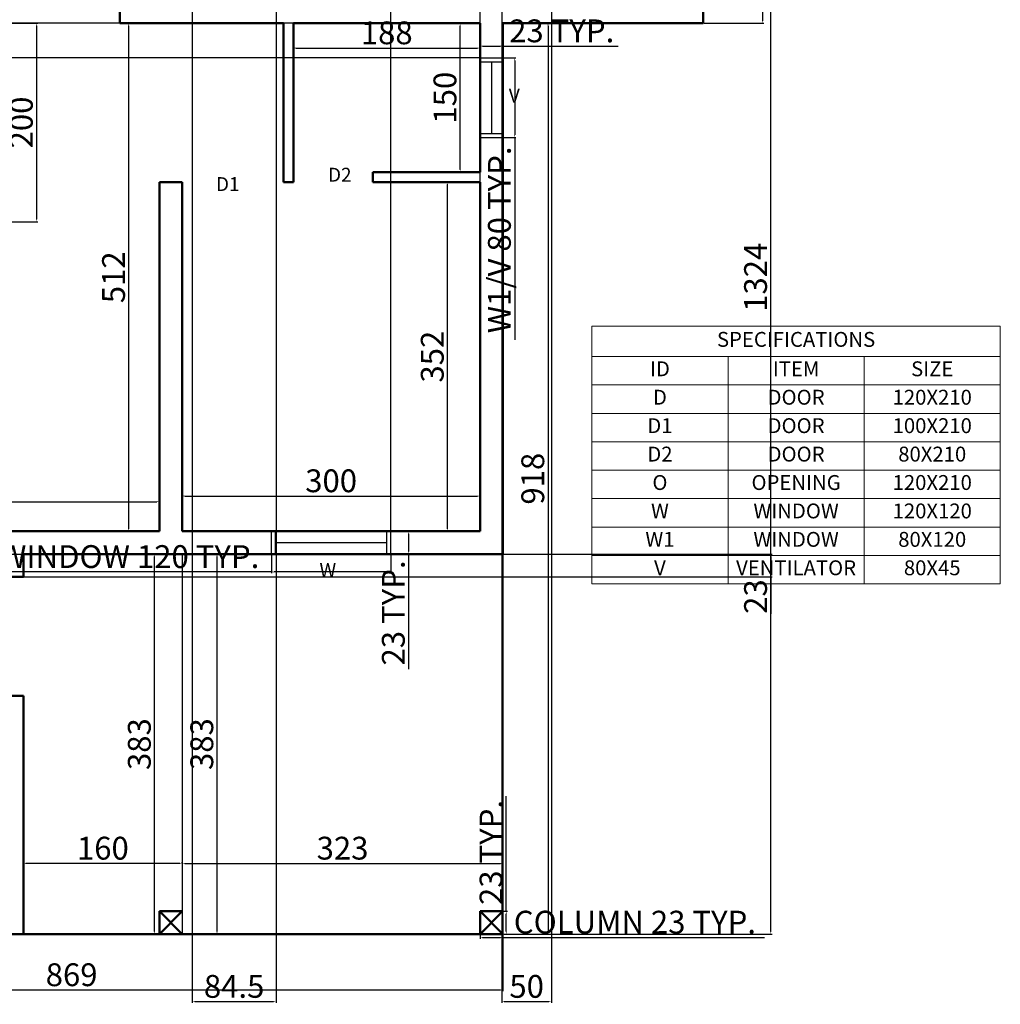
# Model space of a CAD drawing. Units: centimetres. Extents: x 6294 to 7898, y 3240 to 4730.
# Tile 2 of 3: x 6910 to 7898, y 3240 to 4232. Entities that reach past the tile are written whole.
import ezdxf

# ---------------------------------------------------------------- set-up
doc = ezdxf.new("R2010")
doc.units = ezdxf.units.CM
for name, color, linetype, lineweight in [('A-ANNO-DIMS', 2, 'Continuous', 18), ('A-ANNO-SCHD', 7, 'Continuous', 18), ('A-ANNO-TEXT', 7, 'Continuous', 25), ('A-COLS', 7, 'Continuous', 50), ('A-FLOR', 8, 'Continuous', 25), ('A-GLAZ', 4, 'Continuous', 25), ('A-WALL', 7, 'Continuous', 50)]:
    doc.layers.add(name, color=color, linetype=linetype, lineweight=lineweight)
doc.styles.get("Standard").update_dxf_attribs({"font": 'arial.ttf'})
doc.dimstyles.new('ISO-25', dxfattribs={"dimtxt": 23, "dimasz": 2.5, "dimexe": 1.25, "dimexo": 0.625, "dimtad": 1, "dimtxsty": 'Standard', "dimcen": 2.5, "dimadec": 0, "dimazin": 0, "dimtfac": 1, "dimtmove": 0, "dimatfit": 3, "dimfxl": 1, "dimarcsym": 0})

# ---------------------------------------------------------------- blocks, each defined once
blk = doc.blocks.new('*T1')
at = {"layer": 'A-ANNO-SCHD', "transparency": 16777216}
for p, q in [((0, 0), (411.54, 0)), ((0, 0), (0, -259.86)), ((411.54, 0), (411.54, -259.86)), ((0, -30.65), (411.54, -30.65)), ((137.18, -30.65), (137.18, -259.86)), ((274.36, -30.65), (274.36, -259.86)), ((0, -59.3), (411.54, -59.3)), ((0, -87.95), (411.54, -87.95)), ((0, -116.6), (411.54, -116.6)), ((0, -145.25), (411.54, -145.25)), ((0, -173.9), (411.54, -173.9)), ((0, -202.55), (411.54, -202.55)), ((0, -231.2), (411.54, -231.2)), ((0, -259.86), (411.54, -259.86))]:
    blk.add_line(p, q, dxfattribs=at)
at = {"layer": 'A-ANNO-SCHD', "color": 0, "transparency": 16777216, "char_height": 15, "attachment_point": 5}
for s, insert, width in [('SPECIFICATIONS', (205.77, -15.33), 408.5389), ('ID', (68.59, -44.98), 134.1796), ('ITEM', (205.77, -44.98), 134.1796), ('SIZE', (342.95, -44.98), 134.1796), ('D ', (68.59, -73.63), 134.1796), ('DOOR', (205.77, -73.63), 134.1796), ('120X210', (342.95, -73.63), 134.1796), ('D1', (68.59, -102.28), 134.1796), ('DOOR', (205.77, -102.28), 134.1796), ('100X210', (342.95, -102.28), 134.1796), ('D2', (68.59, -130.93), 134.1796), ('DOOR', (205.77, -130.93), 134.1796), ('80X210', (342.95, -130.93), 134.1796), ('O', (68.59, -159.58), 134.1796), ('OPENING', (205.77, -159.58), 134.1796), ('120X210', (342.95, -159.58), 134.1796), ('WINDOW', (205.77, -188.23), 134.1796), ('120X120', (342.95, -188.23), 134.1796), ('W', (68.59, -188.23), 134.1796), ('W1', (68.59, -216.88), 134.1796), ('WINDOW', (205.77, -216.88), 134.1796), ('80X120', (342.95, -216.88), 134.1796), ('V', (68.59, -245.53), 134.1796), ('VENTILATOR', (205.77, -245.53), 134.1796), ('80X45', (342.95, -245.53), 134.1796)]:
    blk.add_mtext(s, dxfattribs=dict(at, insert=insert, width=width))
blk = doc.blocks.new('*D10')
at = {"layer": 'A-ANNO-DIMS', "color": 0, "lineweight": -2, "transparency": 16777216}
for p, q in [((7185.73, 4228.22), (7185.73, 4202.61)), ((7373.73, 4228.22), (7373.73, 4202.61)), ((7188.23, 4203.86), (7371.23, 4203.86))]:
    blk.add_line(p, q, dxfattribs=at)
at = {"layer": 'A-ANNO-DIMS', "color": 0, "transparency": 16777216}
for points in [[(7188.23, 4204.28), (7188.23, 4203.45), (7185.73, 4203.86)], [(7371.23, 4204.28), (7371.23, 4203.45), (7373.73, 4203.86)]]:
    blk.add_solid(points, dxfattribs=at)
at = {"layer": 'Defpoints', "color": 0, "transparency": 16777216}
for p in [(7185.73, 4228.85), (7373.73, 4228.85), (7373.73, 4203.86)]:
    blk.add_point(p, dxfattribs=at)
at = {"layer": 'A-ANNO-DIMS', "color": 0, "transparency": 16777216, "insert": (7279.73, 4216.23), "char_height": 23, "attachment_point": 5}
blk.add_mtext('188', dxfattribs=at)
blk = doc.blocks.new('*D11')
at = {"layer": 'A-ANNO-DIMS', "color": 0, "lineweight": -2, "transparency": 16777216}
for p, q in [((7373.11, 4228.85), (7352.48, 4228.85)), ((7353.73, 4081.35), (7353.73, 4226.35)), ((7373.11, 4078.85), (7352.48, 4078.85))]:
    blk.add_line(p, q, dxfattribs=at)
at = {"layer": 'A-ANNO-DIMS', "color": 0, "transparency": 16777216}
for points in [[(7353.32, 4226.35), (7354.15, 4226.35), (7353.73, 4228.85)], [(7353.32, 4081.35), (7354.15, 4081.35), (7353.73, 4078.85)]]:
    blk.add_solid(points, dxfattribs=at)
at = {"layer": 'Defpoints', "color": 0, "transparency": 16777216}
for p in [(7353.73, 4228.85), (7373.73, 4228.85), (7373.73, 4078.85)]:
    blk.add_point(p, dxfattribs=at)
at = {"layer": 'A-ANNO-DIMS', "color": 0, "transparency": 16777216, "insert": (7341.37, 4153.85), "char_height": 23, "attachment_point": 5, "rotation": 90}
blk.add_mtext('150', dxfattribs=at)
blk = doc.blocks.new('*D12')
at = {"layer": 'A-ANNO-DIMS', "color": 0, "lineweight": -2, "transparency": 16777216}
for p, q in [((7073.73, 3717.47), (7073.73, 3753.63)), ((7076.23, 3752.38), (7371.23, 3752.38)), ((7373.73, 3717.47), (7373.73, 3753.63))]:
    blk.add_line(p, q, dxfattribs=at)
at = {"layer": 'A-ANNO-DIMS', "color": 0, "transparency": 16777216}
for points in [[(7076.23, 3752.8), (7076.23, 3751.96), (7073.73, 3752.38)], [(7371.23, 3752.8), (7371.23, 3751.96), (7373.73, 3752.38)]]:
    blk.add_solid(points, dxfattribs=at)
at = {"layer": 'Defpoints', "color": 0, "transparency": 16777216}
for p in [(7373.73, 3752.38), (7073.73, 3716.85), (7373.73, 3716.85)]:
    blk.add_point(p, dxfattribs=at)
at = {"layer": 'A-ANNO-DIMS', "color": 0, "transparency": 16777216, "insert": (7223.73, 3764.76), "char_height": 23, "attachment_point": 5}
blk.add_mtext('300', dxfattribs=at)
blk = doc.blocks.new('*D13')
at = {"layer": 'A-ANNO-DIMS', "color": 0, "lineweight": -2, "transparency": 16777216}
for p, q in [((7373.11, 4068.85), (7339.75, 4068.85)), ((7341, 3719.35), (7341, 4066.35)), ((7373.11, 3716.85), (7339.75, 3716.85))]:
    blk.add_line(p, q, dxfattribs=at)
at = {"layer": 'A-ANNO-DIMS', "color": 0, "transparency": 16777216}
for points in [[(7340.58, 4066.35), (7341.41, 4066.35), (7341, 4068.85)], [(7340.58, 3719.35), (7341.41, 3719.35), (7341, 3716.85)]]:
    blk.add_solid(points, dxfattribs=at)
at = {"layer": 'Defpoints', "color": 0, "transparency": 16777216}
for p in [(7341, 4068.85), (7373.73, 4068.85), (7373.73, 3716.85)]:
    blk.add_point(p, dxfattribs=at)
at = {"layer": 'A-ANNO-DIMS', "color": 0, "transparency": 16777216, "insert": (7328.62, 3892.85), "char_height": 23, "attachment_point": 5, "rotation": 90}
blk.add_mtext('352', dxfattribs=at)
blk = doc.blocks.new('*D14')
at = {"layer": 'A-ANNO-DIMS', "color": 0, "lineweight": -2, "transparency": 16777216}
for p, q in [((7074.36, 3693.85), (7110.01, 3693.85)), ((7108.76, 3313.35), (7108.76, 3691.35)), ((7074.36, 3310.85), (7110.01, 3310.85))]:
    blk.add_line(p, q, dxfattribs=at)
at = {"layer": 'A-ANNO-DIMS', "color": 0, "transparency": 16777216}
for points in [[(7108.35, 3691.35), (7109.18, 3691.35), (7108.76, 3693.85)], [(7108.35, 3313.35), (7109.18, 3313.35), (7108.76, 3310.85)]]:
    blk.add_solid(points, dxfattribs=at)
at = {"layer": 'Defpoints', "color": 0, "transparency": 16777216}
for p in [(7073.73, 3693.85), (7108.76, 3693.85), (7073.73, 3310.85)]:
    blk.add_point(p, dxfattribs=at)
at = {"layer": 'A-ANNO-DIMS', "color": 0, "transparency": 16777216, "insert": (7096.39, 3502.35), "char_height": 23, "attachment_point": 5, "rotation": 90}
blk.add_mtext('383', dxfattribs=at)
blk = doc.blocks.new('*D15')
at = {"layer": 'A-ANNO-DIMS', "color": 0, "lineweight": -2, "transparency": 16777216}
for p, q in [((7073.73, 3382.75), (7073.73, 3383.37)), ((7076.23, 3382.12), (7394.23, 3382.12)), ((7396.73, 3382.75), (7396.73, 3383.37))]:
    blk.add_line(p, q, dxfattribs=at)
at = {"layer": 'A-ANNO-DIMS', "color": 0, "transparency": 16777216}
for points in [[(7076.23, 3382.54), (7076.23, 3381.71), (7073.73, 3382.12)], [(7394.23, 3382.54), (7394.23, 3381.71), (7396.73, 3382.12)]]:
    blk.add_solid(points, dxfattribs=at)
at = {"layer": 'Defpoints', "color": 0, "transparency": 16777216}
for p in [(7073.73, 3382.12), (7396.73, 3382.12), (7396.73, 3382.12)]:
    blk.add_point(p, dxfattribs=at)
at = {"layer": 'A-ANNO-DIMS', "color": 0, "transparency": 16777216, "insert": (7235.23, 3394.5), "char_height": 23, "attachment_point": 5}
blk.add_mtext('323', dxfattribs=at)
blk = doc.blocks.new('*D16')
at = {"layer": 'A-ANNO-DIMS', "color": 0, "lineweight": -2, "transparency": 16777216}
for p, q in [((6913.73, 3382.75), (6913.73, 3383.37)), ((7071.23, 3382.12), (6916.23, 3382.12)), ((7073.73, 3382.75), (7073.73, 3383.37))]:
    blk.add_line(p, q, dxfattribs=at)
at = {"layer": 'A-ANNO-DIMS', "color": 0, "transparency": 16777216}
for points in [[(6916.23, 3382.54), (6916.23, 3381.71), (6913.73, 3382.12)], [(7071.23, 3382.54), (7071.23, 3381.71), (7073.73, 3382.12)]]:
    blk.add_solid(points, dxfattribs=at)
at = {"layer": 'Defpoints', "color": 0, "transparency": 16777216}
for p in [(6913.73, 3382.12), (6913.73, 3382.12), (7073.73, 3382.12)]:
    blk.add_point(p, dxfattribs=at)
at = {"layer": 'A-ANNO-DIMS', "color": 0, "transparency": 16777216, "insert": (6993.73, 3394.49), "char_height": 23, "attachment_point": 5}
blk.add_mtext('160', dxfattribs=at)
blk = doc.blocks.new('*D17')
at = {"layer": 'A-ANNO-DIMS', "color": 0, "lineweight": -2, "transparency": 16777216}
for p, q in [((7073.11, 3693.85), (7044.56, 3693.85)), ((7045.81, 3313.35), (7045.81, 3691.35)), ((7073.11, 3310.85), (7044.56, 3310.85))]:
    blk.add_line(p, q, dxfattribs=at)
at = {"layer": 'A-ANNO-DIMS', "color": 0, "transparency": 16777216}
for points in [[(7045.4, 3691.35), (7046.23, 3691.35), (7045.81, 3693.85)], [(7045.4, 3313.35), (7046.23, 3313.35), (7045.81, 3310.85)]]:
    blk.add_solid(points, dxfattribs=at)
at = {"layer": 'Defpoints', "color": 0, "transparency": 16777216}
for p in [(7045.81, 3693.85), (7073.73, 3693.85), (7073.73, 3310.85)]:
    blk.add_point(p, dxfattribs=at)
at = {"layer": 'A-ANNO-DIMS', "color": 0, "transparency": 16777216, "insert": (7033.44, 3502.35), "char_height": 23, "attachment_point": 5, "rotation": 90}
blk.add_mtext('383', dxfattribs=at)
blk = doc.blocks.new('*D20')
at = {"layer": 'A-ANNO-DIMS', "color": 0, "lineweight": -2, "transparency": 16777216}
for p, q in [((6550.73, 3717.47), (6550.73, 3747.88)), ((6553.23, 3746.63), (7048.23, 3746.63)), ((7050.73, 3717.47), (7050.73, 3747.88))]:
    blk.add_line(p, q, dxfattribs=at)
at = {"layer": 'A-ANNO-DIMS', "color": 0, "transparency": 16777216}
for points in [[(6553.23, 3747.05), (6553.23, 3746.21), (6550.73, 3746.63)], [(7048.23, 3747.05), (7048.23, 3746.21), (7050.73, 3746.63)]]:
    blk.add_solid(points, dxfattribs=at)
at = {"layer": 'Defpoints', "color": 0, "transparency": 16777216}
for p in [(7050.73, 3746.63), (6550.73, 3716.85), (7050.73, 3716.85)]:
    blk.add_point(p, dxfattribs=at)
at = {"layer": 'A-ANNO-DIMS', "color": 0, "transparency": 16777216, "insert": (6800.73, 3759), "char_height": 23, "attachment_point": 5}
blk.add_mtext('500', dxfattribs=at)
blk = doc.blocks.new('*D21')
at = {"layer": 'A-ANNO-DIMS', "color": 0, "lineweight": -2, "transparency": 16777216}
for p, q in [((7050.11, 4228.85), (7018.56, 4228.85)), ((7019.81, 3719.35), (7019.81, 4226.35)), ((7050.11, 3716.85), (7018.56, 3716.85))]:
    blk.add_line(p, q, dxfattribs=at)
at = {"layer": 'A-ANNO-DIMS', "color": 0, "transparency": 16777216}
for points in [[(7019.39, 4226.35), (7020.22, 4226.35), (7019.81, 4228.85)], [(7019.39, 3719.35), (7020.22, 3719.35), (7019.81, 3716.85)]]:
    blk.add_solid(points, dxfattribs=at)
at = {"layer": 'Defpoints', "color": 0, "transparency": 16777216}
for p in [(7019.81, 4228.85), (7050.73, 4228.85), (7050.73, 3716.85)]:
    blk.add_point(p, dxfattribs=at)
at = {"layer": 'A-ANNO-DIMS', "color": 0, "transparency": 16777216, "insert": (7007.44, 3972.85), "char_height": 23, "attachment_point": 5, "rotation": 90}
blk.add_mtext('512', dxfattribs=at)
blk = doc.blocks.new('*D22')
at = {"layer": 'A-ANNO-DIMS', "color": 0, "lineweight": -2, "transparency": 16777216}
for p, q in [((6891.36, 4228.85), (6928.18, 4228.85)), ((6926.93, 4226.35), (6926.93, 4031.35)), ((6891.36, 4028.85), (6928.18, 4028.85))]:
    blk.add_line(p, q, dxfattribs=at)
at = {"layer": 'A-ANNO-DIMS', "color": 0, "transparency": 16777216}
for points in [[(6926.51, 4226.35), (6927.34, 4226.35), (6926.93, 4228.85)], [(6926.51, 4031.35), (6927.34, 4031.35), (6926.93, 4028.85)]]:
    blk.add_solid(points, dxfattribs=at)
at = {"layer": 'Defpoints', "color": 0, "transparency": 16777216}
for p in [(6890.73, 4228.85), (6890.73, 4028.85), (6926.93, 4028.85)]:
    blk.add_point(p, dxfattribs=at)
at = {"layer": 'A-ANNO-DIMS', "color": 0, "transparency": 16777216, "insert": (6914.56, 4128.85), "char_height": 23, "attachment_point": 5, "rotation": 90}
blk.add_mtext('200', dxfattribs=at)
blk = doc.blocks.new('*D24')
at = {"layer": 'A-ANNO-DIMS', "color": 0, "lineweight": -2, "transparency": 16777216}
for p, q in [((7599.36, 4634.85), (7659.7, 4634.85)), ((7658.45, 4632.35), (7658.45, 4231.35)), ((7599.36, 4228.85), (7659.7, 4228.85))]:
    blk.add_line(p, q, dxfattribs=at)
at = {"layer": 'A-ANNO-DIMS', "color": 0, "transparency": 16777216}
for points in [[(7658.04, 4632.35), (7658.87, 4632.35), (7658.45, 4634.85)], [(7658.04, 4231.35), (7658.87, 4231.35), (7658.45, 4228.85)]]:
    blk.add_solid(points, dxfattribs=at)
at = {"layer": 'Defpoints', "color": 0, "transparency": 16777216}
for p in [(7598.73, 4634.85), (7598.73, 4228.85), (7658.45, 4228.85)]:
    blk.add_point(p, dxfattribs=at)
at = {"layer": 'A-ANNO-DIMS', "color": 0, "transparency": 16777216, "insert": (7646.08, 4431.85), "char_height": 23, "attachment_point": 5, "rotation": 90}
blk.add_mtext('406', dxfattribs=at)
blk = doc.blocks.new('*D25')
at = {"layer": 'A-ANNO-DIMS', "color": 0, "lineweight": -2, "transparency": 16777216}
for p, q in [((7397.36, 4228.85), (7443.5, 4228.85)), ((7442.25, 4226.35), (7442.25, 3313.35)), ((7397.36, 3310.85), (7443.5, 3310.85))]:
    blk.add_line(p, q, dxfattribs=at)
at = {"layer": 'A-ANNO-DIMS', "color": 0, "transparency": 16777216}
for points in [[(7441.83, 4226.35), (7442.67, 4226.35), (7442.25, 4228.85)], [(7441.83, 3313.35), (7442.67, 3313.35), (7442.25, 3310.85)]]:
    blk.add_solid(points, dxfattribs=at)
at = {"layer": 'Defpoints', "color": 0, "transparency": 16777216}
for p in [(7396.73, 4228.85), (7396.73, 3310.85), (7442.25, 3310.85)]:
    blk.add_point(p, dxfattribs=at)
at = {"layer": 'A-ANNO-DIMS', "color": 0, "transparency": 16777216, "insert": (7429.88, 3769.85), "char_height": 23, "attachment_point": 5, "rotation": 90}
blk.add_mtext('918', dxfattribs=at)
blk = doc.blocks.new('*D26')
at = {"layer": 'A-ANNO-DIMS', "color": 0, "lineweight": -2, "transparency": 16777216}
for p, q in [((6527.73, 3310.22), (6527.73, 3253.32)), ((7396.73, 3310.22), (7396.73, 3253.32)), ((6530.23, 3254.57), (7394.23, 3254.57))]:
    blk.add_line(p, q, dxfattribs=at)
at = {"layer": 'A-ANNO-DIMS', "color": 0, "transparency": 16777216}
for points in [[(6530.23, 3254.99), (6530.23, 3254.15), (6527.73, 3254.57)], [(7394.23, 3254.99), (7394.23, 3254.15), (7396.73, 3254.57)]]:
    blk.add_solid(points, dxfattribs=at)
at = {"layer": 'Defpoints', "color": 0, "transparency": 16777216}
for p in [(6527.73, 3310.85), (7396.73, 3310.85), (7396.73, 3254.57)]:
    blk.add_point(p, dxfattribs=at)
at = {"layer": 'A-ANNO-DIMS', "color": 0, "transparency": 16777216, "insert": (6962.23, 3266.94), "char_height": 23, "attachment_point": 5}
blk.add_mtext('869', dxfattribs=at)
blk = doc.blocks.new('WIN-W-120CM')
for p, q in [((0, 23), (0, 0)), ((4, 23), (4, 0)), ((116, 23), (116, 0)), ((120, 23), (120, 0)), ((4, 11.5), (116, 11.5))]:
    blk.add_line(p, q)
blk = doc.blocks.new('FRAME-W1-V-80CM')
for p, q in [((0, 0), (0, 23)), ((4, 0), (4, 23)), ((76, 0), (76, 23)), ((80, 0), (80, 23)), ((4, 11.5), (76, 11.5))]:
    blk.add_line(p, q)
blk = doc.blocks.new('COL-SQUARE-23CM')
for p, q in [((23, 23), (0, 23)), ((0, 23), (0, 0)), ((0, 23), (23, 0)), ((0, 0), (23, 23))]:
    blk.add_line(p, q)
blk = doc.blocks.new('*D32')
at = {"layer": 'A-ANNO-DIMS', "color": 0, "lineweight": -2, "transparency": 16777216}
for p, q in [((7163.73, 3693.22), (7163.73, 3674.6)), ((7283.73, 3693.22), (7283.73, 3674.6)), ((7163.73, 3675.85), (6879.31, 3675.85)), ((7281.23, 3675.85), (7166.23, 3675.85))]:
    blk.add_line(p, q, dxfattribs=at)
at = {"layer": 'A-ANNO-DIMS', "color": 0, "transparency": 16777216}
for points in [[(7166.23, 3676.26), (7166.23, 3675.43), (7163.73, 3675.85)], [(7281.23, 3676.26), (7281.23, 3675.43), (7283.73, 3675.85)]]:
    blk.add_solid(points, dxfattribs=at)
at = {"layer": 'Defpoints', "color": 0, "transparency": 16777216}
for p in [(7163.73, 3693.85), (7283.73, 3693.85), (7163.73, 3675.85)]:
    blk.add_point(p, dxfattribs=at)
at = {"layer": 'A-ANNO-DIMS', "color": 0, "transparency": 16777216, "insert": (7020.27, 3688.37), "char_height": 23, "attachment_point": 5}
blk.add_mtext('WINDOW 120 TYP.', dxfattribs=at)
blk = doc.blocks.new('*D33')
at = {"layer": 'A-ANNO-DIMS', "color": 0, "lineweight": -2, "transparency": 16777216}
for p, q in [((7284.36, 3716.85), (7302.98, 3716.85)), ((7301.73, 3714.35), (7301.73, 3696.35)), ((7284.36, 3693.85), (7302.98, 3693.85)), ((7301.73, 3693.85), (7301.73, 3577.75))]:
    blk.add_line(p, q, dxfattribs=at)
at = {"layer": 'A-ANNO-DIMS', "color": 0, "transparency": 16777216}
for points in [[(7301.32, 3714.35), (7302.15, 3714.35), (7301.73, 3716.85)], [(7301.32, 3696.35), (7302.15, 3696.35), (7301.73, 3693.85)]]:
    blk.add_solid(points, dxfattribs=at)
at = {"layer": 'Defpoints', "color": 0, "transparency": 16777216}
for p in [(7283.73, 3716.85), (7283.73, 3693.85), (7301.73, 3693.85)]:
    blk.add_point(p, dxfattribs=at)
at = {"layer": 'A-ANNO-DIMS', "color": 0, "transparency": 16777216, "insert": (7289.36, 3634.55), "char_height": 23, "attachment_point": 5, "rotation": 90}
blk.add_mtext('23 TYP.', dxfattribs=at)
blk = doc.blocks.new('*D34')
at = {"layer": 'A-ANNO-DIMS', "color": 0, "lineweight": -2, "transparency": 16777216}
for p, q in [((7397.36, 4193.85), (7409.98, 4193.85)), ((7408.73, 4191.35), (7408.73, 4116.35)), ((7397.36, 4113.85), (7409.98, 4113.85)), ((7408.73, 4113.85), (7408.73, 3909.72))]:
    blk.add_line(p, q, dxfattribs=at)
at = {"layer": 'A-ANNO-DIMS', "color": 0, "transparency": 16777216}
for points in [[(7408.32, 4191.35), (7409.15, 4191.35), (7408.73, 4193.85)], [(7408.32, 4116.35), (7409.15, 4116.35), (7408.73, 4113.85)]]:
    blk.add_solid(points, dxfattribs=at)
at = {"layer": 'Defpoints', "color": 0, "transparency": 16777216}
for p in [(7396.73, 4193.85), (7396.73, 4113.85), (7408.73, 4113.85)]:
    blk.add_point(p, dxfattribs=at)
at = {"layer": 'A-ANNO-DIMS', "color": 0, "transparency": 16777216, "insert": (7396.22, 4010.53), "char_height": 23, "attachment_point": 5, "rotation": 90}
blk.add_mtext('W1/V 80 TYP.', dxfattribs=at)
blk = doc.blocks.new('*D35')
at = {"layer": 'A-ANNO-DIMS', "color": 0, "lineweight": -2, "transparency": 16777216}
for p, q in [((7373.73, 4194.47), (7373.73, 4207.1)), ((7376.23, 4205.85), (7394.23, 4205.85)), ((7396.73, 4194.47), (7396.73, 4207.1)), ((7396.73, 4205.85), (7512.83, 4205.85))]:
    blk.add_line(p, q, dxfattribs=at)
at = {"layer": 'A-ANNO-DIMS', "color": 0, "transparency": 16777216}
for points in [[(7376.23, 4206.26), (7376.23, 4205.43), (7373.73, 4205.85)], [(7394.23, 4206.26), (7394.23, 4205.43), (7396.73, 4205.85)]]:
    blk.add_solid(points, dxfattribs=at)
at = {"layer": 'Defpoints', "color": 0, "transparency": 16777216}
for p in [(7396.73, 4205.85), (7373.73, 4193.85), (7396.73, 4193.85)]:
    blk.add_point(p, dxfattribs=at)
at = {"layer": 'A-ANNO-DIMS', "color": 0, "transparency": 16777216, "insert": (7456.03, 4218.22), "char_height": 23, "attachment_point": 5}
blk.add_mtext('23 TYP.', dxfattribs=at)
blk = doc.blocks.new('*D36')
at = {"layer": 'A-ANNO-DIMS', "color": 0, "lineweight": -2, "transparency": 16777216}
for p, q in [((7373.73, 3310.22), (7373.73, 3306.15)), ((7376.23, 3307.4), (7394.23, 3307.4)), ((7396.73, 3310.22), (7396.73, 3306.15)), ((7396.73, 3307.4), (7660.34, 3307.4))]:
    blk.add_line(p, q, dxfattribs=at)
at = {"layer": 'A-ANNO-DIMS', "color": 0, "transparency": 16777216}
for points in [[(7376.23, 3307.81), (7376.23, 3306.98), (7373.73, 3307.4)], [(7394.23, 3307.81), (7394.23, 3306.98), (7396.73, 3307.4)]]:
    blk.add_solid(points, dxfattribs=at)
at = {"layer": 'Defpoints', "color": 0, "transparency": 16777216}
for p in [(7373.73, 3310.85), (7396.73, 3310.85), (7396.73, 3307.4)]:
    blk.add_point(p, dxfattribs=at)
at = {"layer": 'A-ANNO-DIMS', "color": 0, "transparency": 16777216, "insert": (7529.79, 3319.93), "char_height": 23, "attachment_point": 5}
blk.add_mtext('COLUMN 23 TYP.', dxfattribs=at)
blk = doc.blocks.new('*D37')
at = {"layer": 'A-ANNO-DIMS', "color": 0, "lineweight": -2, "transparency": 16777216}
for p, q in [((7400.18, 3333.85), (7400.18, 3449.95)), ((7397.36, 3333.85), (7401.43, 3333.85)), ((7400.18, 3313.35), (7400.18, 3331.35)), ((7397.36, 3310.85), (7401.43, 3310.85))]:
    blk.add_line(p, q, dxfattribs=at)
at = {"layer": 'A-ANNO-DIMS', "color": 0, "transparency": 16777216}
for points in [[(7399.77, 3331.35), (7400.6, 3331.35), (7400.18, 3333.85)], [(7399.77, 3313.35), (7400.6, 3313.35), (7400.18, 3310.85)]]:
    blk.add_solid(points, dxfattribs=at)
at = {"layer": 'Defpoints', "color": 0, "transparency": 16777216}
for p in [(7396.73, 3333.85), (7400.18, 3333.85), (7396.73, 3310.85)]:
    blk.add_point(p, dxfattribs=at)
at = {"layer": 'A-ANNO-DIMS', "color": 0, "transparency": 16777216, "insert": (7387.81, 3393.15), "char_height": 23, "attachment_point": 5, "rotation": 90}
blk.add_mtext('23 TYP.', dxfattribs=at)
blk = doc.blocks.new('*D38')
at = {"layer": 'A-ANNO-DIMS', "color": 0, "lineweight": -2, "transparency": 16777216}
for p, q in [((7599.36, 4634.85), (7667.98, 4634.85)), ((7666.73, 3313.35), (7666.73, 4632.35)), ((7397.36, 3310.85), (7667.98, 3310.85))]:
    blk.add_line(p, q, dxfattribs=at)
at = {"layer": 'A-ANNO-DIMS', "color": 0, "transparency": 16777216}
for points in [[(7666.32, 4632.35), (7667.15, 4632.35), (7666.73, 4634.85)], [(7666.32, 3313.35), (7667.15, 3313.35), (7666.73, 3310.85)]]:
    blk.add_solid(points, dxfattribs=at)
at = {"layer": 'Defpoints', "color": 0, "transparency": 16777216}
for p in [(7598.73, 4634.85), (7666.73, 4634.85), (7396.73, 3310.85)]:
    blk.add_point(p, dxfattribs=at)
at = {"layer": 'A-ANNO-DIMS', "color": 0, "transparency": 16777216, "insert": (7654.36, 3972.85), "char_height": 23, "attachment_point": 5, "rotation": 90}
blk.add_mtext('1324', dxfattribs=at)
blk = doc.blocks.new('*D39')
at = {"layer": 'A-ANNO-DIMS', "color": 0, "lineweight": -2, "transparency": 16777216}
for p, q in [((6404.73, 4129.47), (6404.73, 4704.1)), ((7598.73, 4635.47), (7598.73, 4704.1)), ((6407.23, 4702.85), (7596.23, 4702.85))]:
    blk.add_line(p, q, dxfattribs=at)
at = {"layer": 'A-ANNO-DIMS', "color": 0, "transparency": 16777216}
for points in [[(6407.23, 4703.26), (6407.23, 4702.43), (6404.73, 4702.85)], [(7596.23, 4703.26), (7596.23, 4702.43), (7598.73, 4702.85)]]:
    blk.add_solid(points, dxfattribs=at)
at = {"layer": 'Defpoints', "color": 0, "transparency": 16777216}
for p in [(7598.73, 4702.85), (7598.73, 4634.85), (6404.73, 4128.85)]:
    blk.add_point(p, dxfattribs=at)
at = {"layer": 'A-ANNO-DIMS', "color": 0, "transparency": 16777216, "insert": (7001.73, 4715.22), "char_height": 23, "attachment_point": 5}
blk.add_mtext('1194', dxfattribs=at)
blk = doc.blocks.new('*D40')
at = {"layer": 'A-ANNO-DIMS', "color": 0, "lineweight": -2, "transparency": 16777216}
for p, q in [((6856.73, 4029.47), (6856.73, 4704.1)), ((6890.73, 4029.47), (6890.73, 4704.1)), ((6859.23, 4702.85), (6888.23, 4702.85)), ((6890.73, 4702.85), (6927.32, 4702.85))]:
    blk.add_line(p, q, dxfattribs=at)
at = {"layer": 'A-ANNO-DIMS', "color": 0, "transparency": 16777216}
for points in [[(6859.23, 4703.26), (6859.23, 4702.43), (6856.73, 4702.85)], [(6888.23, 4703.26), (6888.23, 4702.43), (6890.73, 4702.85)]]:
    blk.add_solid(points, dxfattribs=at)
at = {"layer": 'Defpoints', "color": 0, "transparency": 16777216}
for p in [(6890.73, 4702.85), (6856.73, 4028.85), (6890.73, 4028.85)]:
    blk.add_point(p, dxfattribs=at)
at = {"layer": 'A-ANNO-DIMS', "color": 0, "transparency": 16777216, "insert": (6910.28, 4715.22), "char_height": 23, "attachment_point": 5}
blk.add_mtext('34', dxfattribs=at)
blk = doc.blocks.new('*D44')
at = {"layer": 'A-ANNO-DIMS', "color": 0, "lineweight": -2, "transparency": 16777216}
for p, q in [((6891.36, 3693.85), (7667.98, 3693.85)), ((7666.73, 3691.35), (7666.73, 3673.35)), ((6891.36, 3670.85), (7667.98, 3670.85)), ((7666.73, 3670.85), (7666.73, 3633.76))]:
    blk.add_line(p, q, dxfattribs=at)
at = {"layer": 'A-ANNO-DIMS', "color": 0, "transparency": 16777216}
for points in [[(7666.32, 3691.35), (7667.15, 3691.35), (7666.73, 3693.85)], [(7666.32, 3673.35), (7667.15, 3673.35), (7666.73, 3670.85)]]:
    blk.add_solid(points, dxfattribs=at)
at = {"layer": 'Defpoints', "color": 0, "transparency": 16777216}
for p in [(6890.73, 3693.85), (6890.73, 3670.85), (7666.73, 3670.85)]:
    blk.add_point(p, dxfattribs=at)
at = {"layer": 'A-ANNO-DIMS', "color": 0, "transparency": 16777216, "insert": (7654.36, 3651.05), "char_height": 23, "attachment_point": 5, "rotation": 90}
blk.add_mtext('23', dxfattribs=at)
blk = doc.blocks.new('*D46')
at = {"layer": 'A-ANNO-DIMS', "color": 0, "lineweight": -2, "transparency": 16777216}
for p, q in [((7083.73, 4611.22), (7083.73, 3241.6)), ((7168.23, 4611.22), (7168.23, 3241.6)), ((7086.23, 3242.85), (7165.73, 3242.85))]:
    blk.add_line(p, q, dxfattribs=at)
at = {"layer": 'A-ANNO-DIMS', "color": 0, "transparency": 16777216}
for points in [[(7086.23, 3243.26), (7086.23, 3242.43), (7083.73, 3242.85)], [(7165.73, 3243.26), (7165.73, 3242.43), (7168.23, 3242.85)]]:
    blk.add_solid(points, dxfattribs=at)
at = {"layer": 'Defpoints', "color": 0, "transparency": 16777216}
for p in [(7083.73, 4611.85), (7168.23, 4611.85), (7168.23, 3242.85)]:
    blk.add_point(p, dxfattribs=at)
at = {"layer": 'A-ANNO-DIMS', "color": 0, "transparency": 16777216, "insert": (7125.98, 3255.22), "char_height": 23, "attachment_point": 5}
blk.add_mtext('84.5', dxfattribs=at)
blk = doc.blocks.new('*D47')
at = {"layer": 'A-ANNO-DIMS', "color": 0, "lineweight": -2, "transparency": 16777216}
for p, q in [((7395.73, 4611.22), (7395.73, 3241.6)), ((7445.73, 4611.22), (7445.73, 3241.6)), ((7398.23, 3242.85), (7443.23, 3242.85))]:
    blk.add_line(p, q, dxfattribs=at)
at = {"layer": 'A-ANNO-DIMS', "color": 0, "transparency": 16777216}
for points in [[(7398.23, 3243.26), (7398.23, 3242.43), (7395.73, 3242.85)], [(7443.23, 3243.26), (7443.23, 3242.43), (7445.73, 3242.85)]]:
    blk.add_solid(points, dxfattribs=at)
at = {"layer": 'Defpoints', "color": 0, "transparency": 16777216}
for p in [(7395.73, 4611.85), (7445.73, 4611.85), (7445.73, 3242.85)]:
    blk.add_point(p, dxfattribs=at)
at = {"layer": 'A-ANNO-DIMS', "color": 0, "transparency": 16777216, "insert": (7420.73, 3255.22), "char_height": 23, "attachment_point": 5}
blk.add_mtext('50', dxfattribs=at)
blk = doc.blocks.new('*D49')
at = {"layer": 'A-ANNO-DIMS', "color": 0, "lineweight": -2, "transparency": 16777216}
for p, q in [((7373.11, 4228.85), (6335.48, 4228.85)), ((6336.73, 4226.35), (6336.73, 4196.35)), ((7373.11, 4193.85), (6335.48, 4193.85))]:
    blk.add_line(p, q, dxfattribs=at)
at = {"layer": 'A-ANNO-DIMS', "color": 0, "transparency": 16777216}
for points in [[(6336.32, 4226.35), (6337.15, 4226.35), (6336.73, 4228.85)], [(6336.32, 4196.35), (6337.15, 4196.35), (6336.73, 4193.85)]]:
    blk.add_solid(points, dxfattribs=at)
at = {"layer": 'Defpoints', "color": 0, "transparency": 16777216}
for p in [(7373.73, 4228.85), (6336.73, 4193.85), (7373.73, 4193.85)]:
    blk.add_point(p, dxfattribs=at)
at = {"layer": 'A-ANNO-DIMS', "color": 0, "transparency": 16777216, "insert": (6324.36, 4211.35), "char_height": 23, "attachment_point": 5, "rotation": 90}
blk.add_mtext('35', dxfattribs=at)
blk = doc.blocks.new('*D50')
at = {"layer": 'A-ANNO-DIMS', "color": 0, "lineweight": -2, "transparency": 16777216}
for p, q in [((7283.73, 3717.47), (7283.73, 4704.1)), ((7373.73, 3717.47), (7373.73, 4704.1)), ((7371.23, 4702.85), (7286.23, 4702.85))]:
    blk.add_line(p, q, dxfattribs=at)
at = {"layer": 'A-ANNO-DIMS', "color": 0, "transparency": 16777216}
for points in [[(7286.23, 4703.26), (7286.23, 4702.43), (7283.73, 4702.85)], [(7371.23, 4703.26), (7371.23, 4702.43), (7373.73, 4702.85)]]:
    blk.add_solid(points, dxfattribs=at)
at = {"layer": 'Defpoints', "color": 0, "transparency": 16777216}
for p in [(7283.73, 4702.85), (7283.73, 3716.85), (7373.73, 3716.85)]:
    blk.add_point(p, dxfattribs=at)
at = {"layer": 'A-ANNO-DIMS', "color": 0, "transparency": 16777216, "insert": (7328.73, 4715.22), "char_height": 23, "attachment_point": 5}
blk.add_mtext('90', dxfattribs=at)

msp = doc.modelspace()

# ---------------------------------------------------------------- linework, layer by layer
at = {"layer": 'A-FLOR'}
for p, q in [((7073.735, 3693.848), (7073.735, 3310.848)), ((7396.735, 3693.848), (7396.735, 3310.848))]:
    msp.add_line(p, q, dxfattribs=at)
at = {"layer": 'A-WALL'}
for p, q in [((7598.735, 4634.848), (7598.735, 4228.848)), ((7010.735, 4251.848), (7010.735, 4228.848)), ((7175.735, 4228.848), (7010.735, 4228.848)), ((7175.735, 4228.848), (7175.735, 4068.848)), ((7185.735, 4228.848), (7185.735, 4068.848)), ((7373.735, 4228.848), (7185.735, 4228.848)), ((7373.735, 4228.848), (7373.735, 4078.848)), ((7598.735, 4228.848), (7396.735, 4228.848)), ((7396.735, 4228.848), (7396.735, 3693.848)), ((7373.735, 4078.848), (7265.735, 4078.848)), ((7265.735, 4078.848), (7265.735, 4068.848)), ((7050.735, 4068.848), (7050.735, 3716.848)), ((7073.735, 4068.848), (7050.735, 4068.848)), ((7073.735, 4068.848), (7073.735, 3716.848)), ((7185.735, 4068.848), (7175.735, 4068.848)), ((7373.735, 4068.848), (7265.735, 4068.848)), ((7373.735, 4068.848), (7373.735, 3716.848)), ((7050.735, 3716.848), (6780.735, 3716.848)), ((7373.735, 3716.848), (7073.735, 3716.848)), ((7396.735, 3693.848), (6913.735, 3693.848)), ((6913.735, 3693.848), (6913.735, 3670.848)), ((6913.735, 3670.848), (6890.735, 3670.848)), ((6913.735, 3550.848), (6890.735, 3550.848)), ((6913.735, 3550.848), (6913.735, 3310.848)), ((7396.735, 3310.848), (6527.735, 3310.848))]:
    msp.add_line(p, q, dxfattribs=at)

# ---------------------------------------------------------------- block references
msp.add_blockref('*T1', (7486.439, 3923.636))
at = {"layer": 'A-COLS'}
for p in [(7050.735, 3310.848), (7373.735, 3310.848)]:
    msp.add_blockref('COL-SQUARE-23CM', p, dxfattribs=at)
at = {"layer": 'A-GLAZ'}
for name, p, rotation in [('FRAME-W1-V-80CM', (7373.735, 4193.848), 269.9999999999965), ('WIN-W-120CM', (7283.735, 3716.848), 180)]:
    msp.add_blockref(name, p, dxfattribs=dict(at, rotation=rotation))

# ---------------------------------------------------------------- texts
at = {"layer": 'A-ANNO-TEXT'}
for s, height, p in [('V ', 13.9778, (7402.777, 4148.801)), ('D2', 13.9778, (7220.588, 4069.209)), ('D1', 13.9778, (7107.71, 4059.787)), ('W', 13.978, (7211.999, 3670.744))]:
    msp.add_text(s, height=height, dxfattribs=at).set_placement(p)

# ---------------------------------------------------------------- dimensions: what is measured, and where the dimension line sits
at = {"layer": 'A-ANNO-DIMS'}
for base, p1, p2, override, picture, middle in [((7598.735, 4702.848), (6404.735, 4128.848), (7598.735, 4634.848), {"dimdec": 0, "dimlfac": 1, "dimrnd": 0, "dimzin": 0, "dimdsep": 46, "dimlunit": 2}, '*D39', (7001.735, 4715.216)), ((6890.735, 4702.848), (6856.735, 4028.848), (6890.735, 4028.848), {"dimdec": 0, "dimlfac": 1, "dimrnd": 0, "dimzin": 0, "dimdsep": 46, "dimlunit": 2}, '*D40', (6910.278, 4715.224)), ((7283.735, 4702.848), (7373.735, 3716.848), (7283.735, 3716.848), {"dimdec": 0, "dimlfac": 1, "dimrnd": 0, "dimzin": 0, "dimdsep": 46, "dimlunit": 2}, '*D50', (7328.735, 4715.216)), ((7168.235, 3242.848), (7083.735, 4611.848), (7168.235, 4611.848), {"dimdec": 1, "dimlfac": 1, "dimrnd": 0, "dimzin": 0, "dimdsep": 46, "dimlunit": 2}, '*D46', (7125.985, 3255.216)), ((7445.735, 3242.848), (7395.735, 4611.848), (7445.735, 4611.848), {"dimdec": 0, "dimlfac": 1, "dimrnd": 0, "dimzin": 0, "dimdsep": 46, "dimlunit": 2}, '*D47', (7420.735, 3255.216)), ((7373.735, 4203.863), (7185.735, 4228.848), (7373.735, 4228.848), {"dimclrd": 0, "dimclre": 0, "dimclrt": 0}, '*D10', (7279.735, 4216.231)), ((7050.735, 3746.629), (6550.735, 3716.848), (7050.735, 3716.848), {"dimclrd": 0, "dimclre": 0, "dimclrt": 0}, '*D20', (6800.735, 3758.997)), ((7373.735, 3752.381), (7073.735, 3716.848), (7373.735, 3716.848), {"dimclrd": 0, "dimclre": 0, "dimclrt": 0}, '*D12', (7223.735, 3764.757)), ((6913.735, 3382.123), (7073.735, 3382.123), (6913.735, 3382.123), {"dimclrd": 0, "dimclre": 0, "dimclrt": 0}, '*D16', (6993.735, 3394.492)), ((7396.735, 3382.123), (7073.735, 3382.123), (7396.735, 3382.123), {"dimclrd": 0, "dimclre": 0, "dimclrt": 0}, '*D15', (7235.235, 3394.499)), ((7396.735, 3254.57), (6527.735, 3310.848), (7396.735, 3310.848), {"dimclrd": 0, "dimclre": 0, "dimclrt": 0}, '*D26', (6962.235, 3266.938))]:
    dim = msp.add_linear_dim(base=base, p1=p1, p2=p2, dimstyle='ISO-25', override=override, dxfattribs=at)
    dim.commit()
    dim.dimension.update_dxf_attribs({"geometry": picture, "text_midpoint": middle})
for base, p1, p2, angle, override, picture, middle in [((7666.735, 4634.848), (7396.735, 3310.848), (7598.735, 4634.848), 90, {"dimdec": 0, "dimlfac": 1, "dimrnd": 0, "dimzin": 0, "dimdsep": 46, "dimlunit": 2}, '*D38', (7654.359, 3972.848)), ((7658.452, 4228.848), (7598.735, 4634.848), (7598.735, 4228.848), 90, {"dimclrd": 0, "dimclre": 0, "dimclrt": 0}, '*D24', (7646.084, 4431.848)), ((6336.735, 4193.848), (7373.735, 4228.848), (7373.735, 4193.848), 90, {"dimdec": 0, "dimlfac": 1, "dimrnd": 0, "dimzin": 0, "dimdsep": 46, "dimlunit": 2}, '*D49', (6324.359, 4211.348)), ((6926.928, 4028.848), (6890.735, 4228.848), (6890.735, 4028.848), 90, {"dimclrd": 0, "dimclre": 0, "dimclrt": 0}, '*D22', (6914.56, 4128.848)), ((7019.808, 4228.848), (7050.735, 3716.848), (7050.735, 4228.848), 90, {"dimclrd": 0, "dimclre": 0, "dimclrt": 0}, '*D21', (7007.44, 3972.848)), ((7353.733, 4228.848), (7373.735, 4078.848), (7373.735, 4228.848), 270, {"dimclrd": 0, "dimclre": 0, "dimclrt": 0}, '*D11', (7341.365, 4153.848)), ((7442.249, 3310.848), (7396.735, 4228.848), (7396.735, 3310.848), 90, {"dimclrd": 0, "dimclre": 0, "dimclrt": 0}, '*D25', (7429.881, 3769.848)), ((7340.995, 4068.848), (7373.735, 3716.848), (7373.735, 4068.848), 270, {"dimclrd": 0, "dimclre": 0, "dimclrt": 0}, '*D13', (7328.619, 3892.848)), ((7666.735, 3670.848), (6890.735, 3693.848), (6890.735, 3670.848), 90, {"dimdec": 0, "dimlfac": 1, "dimrnd": 0, "dimzin": 0, "dimdsep": 46, "dimlunit": 2}, '*D44', (7654.359, 3651.054)), ((7045.815, 3693.848), (7073.735, 3310.848), (7073.735, 3693.848), 90, {"dimclrd": 0, "dimclre": 0, "dimclrt": 0}, '*D17', (7033.439, 3502.348)), ((7108.764, 3693.848), (7073.735, 3310.848), (7073.735, 3693.848), 270, {"dimclrd": 0, "dimclre": 0, "dimclrt": 0}, '*D14', (7096.388, 3502.348))]:
    dim = msp.add_linear_dim(base=base, p1=p1, p2=p2, angle=angle, dimstyle='ISO-25', override=override, dxfattribs=at)
    dim.commit()
    dim.dimension.update_dxf_attribs({"geometry": picture, "text_midpoint": middle})
for base, p1, p2, text, picture, middle in [((7396.735, 4205.848), (7373.735, 4193.848), (7396.735, 4193.848), '<> TYP.', '*D35', (7456.034, 4218.224)), ((7396.735, 3307.398), (7373.735, 3310.848), (7396.735, 3310.848), 'COLUMN <> TYP.', '*D36', (7529.788, 3319.931))]:
    dim = msp.add_linear_dim(base=base, p1=p1, p2=p2, text=text, dimstyle='ISO-25', override={"dimdec": 0, "dimlfac": 1, "dimrnd": 0, "dimzin": 0, "dimdsep": 46, "dimlunit": 2}, dxfattribs=at)
    dim.commit()
    dim.dimension.update_dxf_attribs({"geometry": picture, "text_midpoint": middle})
for base, p1, p2, angle, text, picture, middle in [((7408.735, 4113.848), (7396.735, 4193.848), (7396.735, 4113.848), 270, 'W1/V <> TYP.', '*D34', (7396.217, 4010.533)), ((7163.735, 3675.848), (7283.735, 3693.848), (7163.735, 3693.848), 180, 'WINDOW <> TYP.', '*D32', (7020.272, 3688.373)), ((7301.735, 3693.848), (7283.735, 3716.848), (7283.735, 3693.848), 270, '<> TYP.', '*D33', (7289.359, 3634.549)), ((7400.185, 3333.848), (7396.735, 3310.848), (7396.735, 3333.848), 90, '<> TYP.', '*D37', (7387.809, 3393.147))]:
    dim = msp.add_linear_dim(base=base, p1=p1, p2=p2, angle=angle, text=text, dimstyle='ISO-25', override={"dimdec": 0, "dimlfac": 1, "dimrnd": 0, "dimzin": 0, "dimdsep": 46, "dimlunit": 2}, dxfattribs=at)
    dim.commit()
    dim.dimension.update_dxf_attribs({"geometry": picture, "text_midpoint": middle})

doc.saveas('drawing.dxf')
